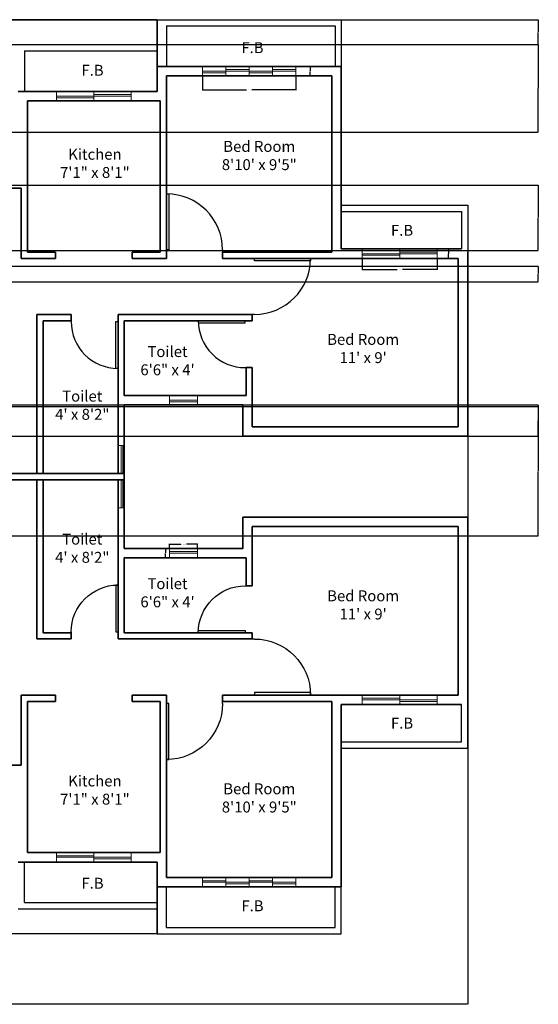
# Model space of a CAD drawing. Units: feet. Extents: x 105 to 1094, y -88 to 588.
# Tile 59 of 59: x 762 to 1094, y -88 to 543. Entities that reach past the tile are written whole.
import ezdxf

# ---------------------------------------------------------------- set-up
doc = ezdxf.new("R2010")
doc.units = ezdxf.units.FT
doc.header["$MEASUREMENT"] = 0
for name, color, linetype, lineweight in [('A-ANNO-DIMS', 2, 'Continuous', 18), ('A-ANNO-TEXT', 7, 'Continuous', 18), ('A-AREA-IDEN', 7, 'Continuous', 18), ('A-DOOR', 3, 'Continuous', 25), ('A-FLOR-PROJ', 8, 'Continuous', 25), ('A-GLAZ', 4, 'Continuous', 18), ('A-WALL', 7, 'Continuous', 35)]:
    doc.layers.add(name, color=color, linetype=linetype, lineweight=lineweight)
doc.styles.get("Standard").update_dxf_attribs({"font": 'arial.ttf'})
doc.dimstyles.get("Standard").update_dxf_attribs({"dimtxt": 0.18, "dimasz": 0.18, "dimexe": 0.18, "dimexo": 0.0625, "dimgap": 0.09, "dimtad": 0, "dimtih": 1, "dimtoh": 1, "dimdec": 4, "dimzin": 0, "dimdsep": 46, "dimtxsty": 'Standard', "dimcen": 0.09, "dimadec": 0, "dimazin": 0, "dimtfac": 1, "dimtdec": 4, "dimtofl": 0, "dimtmove": 0, "dimatfit": 3, "dimfxl": 1, "dimtolj": 1, "dimtzin": 0, "dimarcsym": 0})

# ---------------------------------------------------------------- blocks, each defined once
blk = doc.blocks.new('*U2')
for p, q in [((0, 0), (0, -6)), ((40, 0), (40, -6))]:
    blk.add_line(p, q)
blk.add_lwpolyline([(0, 0), (0, 40), (1.75, 40), (1.75, 0)], close=True)
blk.add_arc((0, 0), 40, 0, 90)
blk = doc.blocks.new('*U4')
for p, q in [((0, 0), (0, -6)), ((-40, 0), (-40, -6))]:
    blk.add_line(p, q)
blk.add_lwpolyline([(0, 0), (0, 40), (-1.75, 40), (-1.75, 0)], close=True)
blk.add_arc((0, 0), 40, 90, 180)
blk = doc.blocks.new('WIN-TWO-LIGHT')
for p, q in [((0, 0), (0, 6)), ((0, 3), (48, 3)), ((0, 2), (24, 2)), ((24, 0), (24, 6)), ((24, 4), (48, 4)), ((48, 0), (48, 6))]:
    blk.add_line(p, q)
blk = doc.blocks.new('WIN-FOUR-LIGHT')
for p, q in [((0, 0), (0, 6)), ((0, 3), (60, 3)), ((0, 2), (15, 2)), ((15, 0), (15, 6)), ((15, 4), (30, 4)), ((30, 0), (30, 6)), ((30, 2), (45, 2)), ((45, 0), (45, 6)), ((45, 4), (60, 4)), ((60, 0), (60, 6))]:
    blk.add_line(p, q)
blk = doc.blocks.new('VENT-TRANSVERSE')
for p, q in [((0, 0), (0, 6)), ((0, 3), (18, 3)), ((0, 2), (18, 2)), ((18, 0), (18, 6))]:
    blk.add_line(p, q)
blk = doc.blocks.new('VENT-LONGITUDINAL')
for p, q in [((0, 18), (4, 18)), ((2.04, 0), (2, 18)), ((3.04, 0), (3, 18))]:
    blk.add_line(p, q)
blk = doc.blocks.new('*D10')
at = {"layer": 'A-ANNO-DIMS', "color": 0, "lineweight": -2, "transparency": 16777216}
for p, q in [((981.19, 390.02), (981.19, 382.7)), ((1029.19, 390.02), (1029.19, 382.7)), ((981.37, 382.88), (1003.56, 382.88)), ((1029.01, 382.88), (1006.82, 382.88))]:
    blk.add_line(p, q, dxfattribs=at)
at = {"layer": 'A-ANNO-DIMS', "color": 0, "transparency": 16777216}
for points in [[(981.37, 382.91), (981.37, 382.85), (981.19, 382.88)], [(1029.01, 382.91), (1029.01, 382.85), (1029.19, 382.88)]]:
    blk.add_solid(points, dxfattribs=at)
at = {"layer": 'Defpoints', "color": 0, "transparency": 16777216}
for p in [(981.19, 390.08), (1029.19, 390.08), (981.19, 382.88)]:
    blk.add_point(p, dxfattribs=at)
at = {"layer": 'A-ANNO-DIMS', "color": 0, "transparency": 16777216, "insert": (1005.19, 382.88), "char_height": 0.18, "attachment_point": 5}
blk.add_mtext('\\A1;2-LIGHT WINDOW 48 TYP.', dxfattribs=at)
blk = doc.blocks.new('*D11')
at = {"layer": 'A-ANNO-DIMS', "color": 0, "lineweight": -2, "transparency": 16777216}
for p, q in [((1029.25, 396.08), (1036.57, 396.08)), ((1036.39, 395.9), (1036.39, 393.26)), ((1036.39, 390.26), (1036.39, 392.9)), ((1029.25, 390.08), (1036.57, 390.08))]:
    blk.add_line(p, q, dxfattribs=at)
at = {"layer": 'A-ANNO-DIMS', "color": 0, "transparency": 16777216}
for points in [[(1036.36, 395.9), (1036.42, 395.9), (1036.39, 396.08)], [(1036.36, 390.26), (1036.42, 390.26), (1036.39, 390.08)]]:
    blk.add_solid(points, dxfattribs=at)
at = {"layer": 'Defpoints', "color": 0, "transparency": 16777216}
for p in [(1029.19, 396.08), (1029.19, 390.08), (1036.39, 390.08)]:
    blk.add_point(p, dxfattribs=at)
at = {"layer": 'A-ANNO-DIMS', "color": 0, "transparency": 16777216, "insert": (1036.39, 393.08), "char_height": 0.18, "attachment_point": 5}
blk.add_mtext('\\A1;6 TYP.', dxfattribs=at)
blk = doc.blocks.new('*D14')
at = {"layer": 'A-ANNO-DIMS', "color": 0, "lineweight": -2, "transparency": 16777216}
for p, q in [((878.69, 507.02), (878.69, 497.9)), ((938.69, 507.02), (938.69, 497.9)), ((878.87, 498.08), (907.05, 498.08)), ((938.51, 498.08), (910.32, 498.08))]:
    blk.add_line(p, q, dxfattribs=at)
at = {"layer": 'A-ANNO-DIMS', "color": 0, "transparency": 16777216}
for points in [[(878.87, 498.11), (878.87, 498.05), (878.69, 498.08)], [(938.51, 498.11), (938.51, 498.05), (938.69, 498.08)]]:
    blk.add_solid(points, dxfattribs=at)
at = {"layer": 'Defpoints', "color": 0, "transparency": 16777216}
for p in [(878.69, 507.08), (938.69, 507.08), (938.69, 498.08)]:
    blk.add_point(p, dxfattribs=at)
at = {"layer": 'A-ANNO-DIMS', "color": 0, "transparency": 16777216, "insert": (908.69, 498.08), "char_height": 0.18, "attachment_point": 5}
blk.add_mtext('\\A1;4-LIGHT WINDOW 60 TYP.', dxfattribs=at)
blk = doc.blocks.new('*D15')
at = {"layer": 'A-ANNO-DIMS', "color": 0, "lineweight": -2, "transparency": 16777216}
for p, q in [((938.75, 513.08), (947.87, 513.08)), ((947.69, 512.9), (947.69, 510.26)), ((938.75, 507.08), (947.87, 507.08)), ((947.69, 507.26), (947.69, 509.9))]:
    blk.add_line(p, q, dxfattribs=at)
at = {"layer": 'A-ANNO-DIMS', "color": 0, "transparency": 16777216}
for points in [[(947.66, 512.9), (947.72, 512.9), (947.69, 513.08)], [(947.66, 507.26), (947.72, 507.26), (947.69, 507.08)]]:
    blk.add_solid(points, dxfattribs=at)
at = {"layer": 'Defpoints', "color": 0, "transparency": 16777216}
for p in [(938.69, 513.08), (947.69, 513.08), (938.69, 507.08)]:
    blk.add_point(p, dxfattribs=at)
at = {"layer": 'A-ANNO-DIMS', "color": 0, "transparency": 16777216, "insert": (947.69, 510.08), "char_height": 0.18, "attachment_point": 5}
blk.add_mtext('\\A1;6 TYP.', dxfattribs=at)
blk = doc.blocks.new('*D16')
at = {"layer": 'A-ANNO-DIMS', "color": 0, "lineweight": -2, "transparency": 16777216}
for p, q in [((857.69, 204.14), (857.69, 206.96)), ((857.87, 206.78), (864.9, 206.78)), ((875.51, 206.78), (868.48, 206.78)), ((875.69, 204.14), (875.69, 206.96))]:
    blk.add_line(p, q, dxfattribs=at)
at = {"layer": 'A-ANNO-DIMS', "color": 0, "transparency": 16777216}
for points in [[(857.87, 206.81), (857.87, 206.75), (857.69, 206.78)], [(875.51, 206.81), (875.51, 206.75), (875.69, 206.78)]]:
    blk.add_solid(points, dxfattribs=at)
at = {"layer": 'Defpoints', "color": 0, "transparency": 16777216}
for p in [(857.69, 206.78), (857.69, 204.08), (875.69, 204.08)]:
    blk.add_point(p, dxfattribs=at)
at = {"layer": 'A-ANNO-DIMS', "color": 0, "transparency": 16777216, "insert": (866.69, 206.78), "char_height": 0.18, "attachment_point": 5}
blk.add_mtext('\\A1;TRANSVERSE VENT 18 TYP.', dxfattribs=at)
blk = doc.blocks.new('*D17')
at = {"layer": 'A-ANNO-DIMS', "color": 0, "lineweight": -2, "transparency": 16777216}
for p, q in [((857.63, 204.08), (854.81, 204.08)), ((854.99, 203.9), (854.99, 201.26)), ((857.63, 198.08), (854.81, 198.08)), ((854.99, 198.26), (854.99, 200.9))]:
    blk.add_line(p, q, dxfattribs=at)
at = {"layer": 'A-ANNO-DIMS', "color": 0, "transparency": 16777216}
for points in [[(854.96, 203.9), (855.02, 203.9), (854.99, 204.08)], [(854.96, 198.26), (855.02, 198.26), (854.99, 198.08)]]:
    blk.add_solid(points, dxfattribs=at)
at = {"layer": 'Defpoints', "color": 0, "transparency": 16777216}
for p in [(857.69, 204.08), (854.99, 198.08), (857.69, 198.08)]:
    blk.add_point(p, dxfattribs=at)
at = {"layer": 'A-ANNO-DIMS', "color": 0, "transparency": 16777216, "insert": (854.99, 201.08), "char_height": 0.18, "attachment_point": 5}
blk.add_mtext('\\A1;6 TYP.', dxfattribs=at)
blk = doc.blocks.new('*D20')
at = {"layer": 'A-ANNO-DIMS', "color": 0, "lineweight": -2, "transparency": 16777216}
for p, q in [((150.69, 276.02), (150.69, -88.15)), ((1048.69, 276.02), (1048.69, -88.15)), ((150.87, -87.97), (599.4, -87.97)), ((1048.51, -87.97), (599.98, -87.97))]:
    blk.add_line(p, q, dxfattribs=at)
at = {"layer": 'A-ANNO-DIMS', "color": 0, "transparency": 16777216}
for points in [[(150.87, -87.94), (150.87, -88), (150.69, -87.97)], [(1048.51, -87.94), (1048.51, -88), (1048.69, -87.97)]]:
    blk.add_solid(points, dxfattribs=at)
at = {"layer": 'Defpoints', "color": 0, "transparency": 16777216}
for p in [(150.69, 276.08), (1048.69, 276.08), (1048.69, -87.97)]:
    blk.add_point(p, dxfattribs=at)
at = {"layer": 'A-ANNO-DIMS', "color": 0, "transparency": 16777216, "insert": (599.69, -87.97), "char_height": 0.18, "attachment_point": 5}
blk.add_mtext('\\A1;898', dxfattribs=at)
blk = doc.blocks.new('*D21')
at = {"layer": 'A-ANNO-DIMS', "color": 0, "lineweight": -2, "transparency": 16777216}
for p, q in [((849.63, 543.08), (105.46, 543.08)), ((105.64, 542.9), (105.64, 250.26)), ((105.64, -42.74), (105.64, 249.9)), ((849.63, -42.92), (105.46, -42.92))]:
    blk.add_line(p, q, dxfattribs=at)
at = {"layer": 'A-ANNO-DIMS', "color": 0, "transparency": 16777216}
for points in [[(105.61, 542.9), (105.67, 542.9), (105.64, 543.08)], [(105.61, -42.74), (105.67, -42.74), (105.64, -42.92)]]:
    blk.add_solid(points, dxfattribs=at)
at = {"layer": 'Defpoints', "color": 0, "transparency": 16777216}
for p in [(105.64, 543.08), (849.69, 543.08), (849.69, -42.92)]:
    blk.add_point(p, dxfattribs=at)
at = {"layer": 'A-ANNO-DIMS', "color": 0, "transparency": 16777216, "insert": (105.64, 250.08), "char_height": 0.18, "attachment_point": 5}
blk.add_mtext('\\A1;586', dxfattribs=at)
blk = doc.blocks.new('*D30')
at = {"layer": 'A-ANNO-DIMS', "color": 0, "lineweight": -2, "transparency": 16777216}
for p, q in [((349.75, 543.08), (1093.92, 543.08)), ((1093.74, 542.9), (1093.74, 535.26)), ((1093.74, 527.26), (1093.74, 534.9)), ((349.75, 527.08), (1093.92, 527.08))]:
    blk.add_line(p, q, dxfattribs=at)
at = {"layer": 'A-ANNO-DIMS', "color": 0, "transparency": 16777216}
for points in [[(1093.71, 542.9), (1093.77, 542.9), (1093.74, 543.08)], [(1093.71, 527.26), (1093.77, 527.26), (1093.74, 527.08)]]:
    blk.add_solid(points, dxfattribs=at)
at = {"layer": 'Defpoints', "color": 0, "transparency": 16777216}
for p in [(349.69, 543.08), (349.69, 527.08), (1093.74, 527.08)]:
    blk.add_point(p, dxfattribs=at)
at = {"layer": 'A-ANNO-DIMS', "color": 0, "transparency": 16777216, "insert": (1093.74, 535.08), "char_height": 0.18, "attachment_point": 5}
blk.add_mtext('\\A1;16', dxfattribs=at)
blk = doc.blocks.new('*D31')
at = {"layer": 'A-ANNO-DIMS', "color": 0, "lineweight": -2, "transparency": 16777216}
for p, q in [((438.75, 527.08), (1093.92, 527.08)), ((1093.74, 526.9), (1093.74, 499.26)), ((1093.74, 471.26), (1093.74, 498.9)), ((438.75, 471.08), (1093.92, 471.08))]:
    blk.add_line(p, q, dxfattribs=at)
at = {"layer": 'A-ANNO-DIMS', "color": 0, "transparency": 16777216}
for points in [[(1093.71, 526.9), (1093.77, 526.9), (1093.74, 527.08)], [(1093.71, 471.26), (1093.77, 471.26), (1093.74, 471.08)]]:
    blk.add_solid(points, dxfattribs=at)
at = {"layer": 'Defpoints', "color": 0, "transparency": 16777216}
for p in [(438.69, 527.08), (1093.74, 527.08), (438.69, 471.08)]:
    blk.add_point(p, dxfattribs=at)
at = {"layer": 'A-ANNO-DIMS', "color": 0, "transparency": 16777216, "insert": (1093.74, 499.08), "char_height": 0.18, "attachment_point": 5}
blk.add_mtext('\\A1;56', dxfattribs=at)
blk = doc.blocks.new('*D34')
at = {"layer": 'A-ANNO-DIMS', "color": 0, "lineweight": -2, "transparency": 16777216}
for p, q in [((552.75, 295.08), (1093.92, 295.08)), ((1093.74, 294.9), (1093.74, 253.76)), ((1093.74, 212.26), (1093.74, 253.4)), ((552.75, 212.08), (1093.92, 212.08))]:
    blk.add_line(p, q, dxfattribs=at)
at = {"layer": 'A-ANNO-DIMS', "color": 0, "transparency": 16777216}
for points in [[(1093.71, 294.9), (1093.77, 294.9), (1093.74, 295.08)], [(1093.71, 212.26), (1093.77, 212.26), (1093.74, 212.08)]]:
    blk.add_solid(points, dxfattribs=at)
at = {"layer": 'Defpoints', "color": 0, "transparency": 16777216}
for p in [(552.69, 295.08), (552.69, 212.08), (1093.74, 212.08)]:
    blk.add_point(p, dxfattribs=at)
at = {"layer": 'A-ANNO-DIMS', "color": 0, "transparency": 16777216, "insert": (1093.74, 253.58), "char_height": 0.18, "attachment_point": 5}
blk.add_mtext('\\A1;83', dxfattribs=at)
blk = doc.blocks.new('*D45')
at = {"layer": 'A-ANNO-DIMS', "color": 0, "lineweight": -2, "transparency": 16777216}
for p, q in [((552.75, 437.08), (1093.92, 437.08)), ((1093.74, 436.9), (1093.74, 416.26)), ((1093.74, 395.26), (1093.74, 415.9)), ((552.75, 395.08), (1093.92, 395.08))]:
    blk.add_line(p, q, dxfattribs=at)
at = {"layer": 'A-ANNO-DIMS', "color": 0, "transparency": 16777216}
for points in [[(1093.71, 436.9), (1093.77, 436.9), (1093.74, 437.08)], [(1093.71, 395.26), (1093.77, 395.26), (1093.74, 395.08)]]:
    blk.add_solid(points, dxfattribs=at)
at = {"layer": 'Defpoints', "color": 0, "transparency": 16777216}
for p in [(552.69, 437.08), (552.69, 395.08), (1093.74, 395.08)]:
    blk.add_point(p, dxfattribs=at)
at = {"layer": 'A-ANNO-DIMS', "color": 0, "transparency": 16777216, "insert": (1093.74, 416.08), "char_height": 0.18, "attachment_point": 5}
blk.add_mtext('\\A1;42', dxfattribs=at)
blk = doc.blocks.new('*D50')
at = {"layer": 'A-ANNO-DIMS', "color": 0, "lineweight": -2, "transparency": 16777216}
for p, q in [((552.75, 385.08), (1093.92, 385.08)), ((1093.74, 384.9), (1093.74, 380.26)), ((1093.74, 375.26), (1093.74, 379.9)), ((552.75, 375.08), (1093.92, 375.08))]:
    blk.add_line(p, q, dxfattribs=at)
at = {"layer": 'A-ANNO-DIMS', "color": 0, "transparency": 16777216}
for points in [[(1093.71, 384.9), (1093.77, 384.9), (1093.74, 385.08)], [(1093.71, 375.26), (1093.77, 375.26), (1093.74, 375.08)]]:
    blk.add_solid(points, dxfattribs=at)
at = {"layer": 'Defpoints', "color": 0, "transparency": 16777216}
for p in [(552.69, 385.08), (552.69, 375.08), (1093.74, 375.08)]:
    blk.add_point(p, dxfattribs=at)
at = {"layer": 'A-ANNO-DIMS', "color": 0, "transparency": 16777216, "insert": (1093.74, 380.08), "char_height": 0.18, "attachment_point": 5}
blk.add_mtext('\\A1;10', dxfattribs=at)
blk = doc.blocks.new('*D54')
at = {"layer": 'A-ANNO-DIMS', "color": 0, "lineweight": -2, "transparency": 16777216}
for p, q in [((294.75, 296.08), (1093.92, 296.08)), ((1093.74, 295.9), (1093.74, 286.26)), ((1093.74, 276.26), (1093.74, 285.9)), ((294.75, 276.08), (1093.92, 276.08))]:
    blk.add_line(p, q, dxfattribs=at)
at = {"layer": 'A-ANNO-DIMS', "color": 0, "transparency": 16777216}
for points in [[(1093.71, 295.9), (1093.77, 295.9), (1093.74, 296.08)], [(1093.71, 276.26), (1093.77, 276.26), (1093.74, 276.08)]]:
    blk.add_solid(points, dxfattribs=at)
at = {"layer": 'Defpoints', "color": 0, "transparency": 16777216}
for p in [(294.69, 296.08), (1093.74, 296.08), (294.69, 276.08)]:
    blk.add_point(p, dxfattribs=at)
at = {"layer": 'A-ANNO-DIMS', "color": 0, "transparency": 16777216, "insert": (1093.74, 286.08), "char_height": 0.18, "attachment_point": 5}
blk.add_mtext('\\A1;20', dxfattribs=at)

msp = doc.modelspace()

# ---------------------------------------------------------------- linework, layer by layer
at = {"layer": 'A-FLOR-PROJ'}
for p, q in [((849.6883, 543.0812), (967.6883, 543.0812)), ((967.6883, 543.0812), (967.6883, 513.0812)), ((855.6883, 539.0812), (855.6883, 513.0812)), ((855.6883, 539.0812), (963.6883, 539.0812)), ((963.6883, 539.0812), (963.6883, 513.0812)), ((760.6883, 527.0812), (849.6883, 527.0812)), ((855.6883, 527.0812), (855.6883, 513.0812)), ((764.6883, 523.0812), (849.6883, 523.0812)), ((764.6883, 523.0812), (764.6883, 497.0812)), ((967.6883, 424.0812), (1048.6883, 424.0812)), ((1048.6883, 424.0812), (1048.6883, 394.0812)), ((967.6883, 420.0812), (1044.6883, 420.0812)), ((1044.6883, 420.0812), (1044.6883, 396.0812)), ((1044.6883, 80.0812), (1044.6883, 104.0812)), ((1048.6883, 76.0812), (1048.6883, 106.0812)), ((967.6883, 80.0812), (1044.6883, 80.0812)), ((967.6883, 76.0812), (1048.6883, 76.0812)), ((764.6883, -22.9188), (764.6883, 3.0812)), ((855.6883, -38.9188), (855.6883, -12.9188)), ((855.6883, -26.9188), (855.6883, -12.9188)), ((963.6883, -38.9188), (963.6883, -12.9188)), ((967.6883, -42.9188), (967.6883, -12.9188)), ((764.6883, -22.9188), (849.6883, -22.9188)), ((760.6883, -26.9188), (849.6883, -26.9188)), ((849.6883, -42.9188), (967.6883, -42.9188)), ((855.6883, -38.9188), (963.6883, -38.9188))]:
    msp.add_line(p, q, dxfattribs=at)
at = {"layer": 'A-WALL'}
for p, q in [((849.6883, 543.0812), (849.6883, 497.0812)), ((849.6883, 513.0812), (967.6883, 513.0812)), ((967.6883, 513.0812), (967.6883, 396.0812)), ((855.6883, 507.0812), (855.6883, 390.0812)), ((855.6883, 507.0812), (961.6883, 507.0812)), ((961.6883, 507.0812), (961.6883, 394.0812)), ((760.6883, 497.0812), (849.6883, 497.0812)), ((766.6883, 491.0812), (766.6883, 394.0812)), ((766.6883, 491.0812), (851.6883, 491.0812)), ((851.6883, 491.0812), (851.6883, 394.0812)), ((762.6883, 435.0812), (652.6883, 435.0812)), ((762.6883, 435.0812), (762.6883, 390.0812)), ((766.6883, 394.0812), (784.6883, 394.0812)), ((784.6883, 394.0812), (784.6883, 390.0812)), ((833.6883, 394.0812), (833.6883, 390.0812)), ((833.6883, 394.0812), (851.6883, 394.0812)), ((891.6883, 394.0812), (891.6883, 390.0812)), ((891.6883, 394.0812), (961.6883, 394.0812)), ((967.6883, 396.0812), (1044.6883, 396.0812)), ((1048.6883, 276.0812), (1048.6883, 394.0812)), ((762.6883, 390.0812), (784.6883, 390.0812)), ((833.6883, 390.0812), (855.6883, 390.0812)), ((891.6883, 390.0812), (1042.6883, 390.0812)), ((1042.6883, 282.0812), (1042.6883, 390.0812)), ((772.6883, 252.0812), (772.6883, 354.0812)), ((772.6883, 354.0812), (794.6883, 354.0812)), ((794.6883, 350.0812), (794.6883, 354.0812)), ((824.6883, 252.0812), (824.6883, 354.0812)), ((824.6883, 354.0812), (910.6883, 354.0812)), ((910.6883, 350.0812), (910.6883, 354.0812)), ((776.6883, 252.0812), (776.6883, 350.0812)), ((776.6883, 350.0812), (794.6883, 350.0812)), ((828.6883, 302.0812), (828.6883, 350.0812)), ((828.6883, 350.0812), (910.6883, 350.0812)), ((906.6883, 302.0812), (906.6883, 320.0812)), ((906.6883, 320.0812), (910.6883, 320.0812)), ((910.6883, 282.0812), (910.6883, 320.0812)), ((828.6883, 302.0812), (906.6883, 302.0812)), ((828.6883, 248.0812), (828.6883, 296.0812)), ((828.6883, 296.0812), (904.6883, 296.0812)), ((904.6883, 276.0812), (904.6883, 296.0812)), ((910.6883, 282.0812), (1042.6883, 282.0812)), ((904.6883, 276.0812), (1048.6883, 276.0812)), ((646.6883, 252.0812), (772.6883, 252.0812)), ((646.6883, 252.0812), (828.6883, 252.0812)), ((646.6883, 248.0812), (828.6883, 248.0812)), ((646.6883, 248.0812), (772.6883, 248.0812)), ((772.6883, 248.0812), (772.6883, 146.0812)), ((776.6883, 252.0812), (828.6883, 252.0812)), ((776.6883, 248.0812), (828.6883, 248.0812)), ((776.6883, 248.0812), (776.6883, 150.0812)), ((824.6883, 248.0812), (824.6883, 146.0812)), ((828.6883, 252.0812), (828.6883, 204.0812)), ((904.6883, 224.0812), (1048.6883, 224.0812)), ((904.6883, 224.0812), (904.6883, 204.0812)), ((1048.6883, 224.0812), (1048.6883, 106.0812)), ((910.6883, 218.0812), (1042.6883, 218.0812)), ((910.6883, 218.0812), (910.6883, 180.0812)), ((1042.6883, 218.0812), (1042.6883, 110.0812)), ((828.6883, 204.0812), (904.6883, 204.0812)), ((828.6883, 198.0812), (906.6883, 198.0812)), ((828.6883, 198.0812), (828.6883, 150.0812)), ((906.6883, 198.0812), (906.6883, 180.0812)), ((906.6883, 180.0812), (910.6883, 180.0812)), ((772.6883, 146.0812), (794.6883, 146.0812)), ((776.6883, 150.0812), (794.6883, 150.0812)), ((794.6883, 150.0812), (794.6883, 146.0812)), ((824.6883, 146.0812), (910.6883, 146.0812)), ((828.6883, 150.0812), (910.6883, 150.0812)), ((910.6883, 150.0812), (910.6883, 146.0812)), ((762.6883, 110.0812), (784.6883, 110.0812)), ((762.6883, 65.0812), (762.6883, 110.0812)), ((784.6883, 106.0812), (784.6883, 110.0812)), ((833.6883, 110.0812), (855.6883, 110.0812)), ((833.6883, 106.0812), (833.6883, 110.0812)), ((855.6883, -6.9188), (855.6883, 110.0812)), ((891.6883, 110.0812), (1042.6883, 110.0812)), ((891.6883, 106.0812), (891.6883, 110.0812)), ((766.6883, 106.0812), (784.6883, 106.0812)), ((766.6883, 9.0812), (766.6883, 106.0812)), ((833.6883, 106.0812), (851.6883, 106.0812)), ((851.6883, 9.0812), (851.6883, 106.0812)), ((891.6883, 106.0812), (961.6883, 106.0812)), ((961.6883, -6.9188), (961.6883, 106.0812)), ((967.6883, 104.0812), (1044.6883, 104.0812)), ((967.6883, -12.9188), (967.6883, 104.0812)), ((762.6883, 65.0812), (652.6883, 65.0812)), ((766.6883, 9.0812), (851.6883, 9.0812)), ((760.6883, 3.0812), (849.6883, 3.0812)), ((849.6883, -42.9188), (849.6883, 3.0812)), ((855.6883, -6.9188), (961.6883, -6.9188)), ((849.6883, -12.9188), (967.6883, -12.9188))]:
    msp.add_line(p, q, dxfattribs=at)

# ---------------------------------------------------------------- block references
at = {"layer": 'A-DOOR'}
for p, xscale, yscale, zscale in [((855.6883, 395.4719), 0.8984622266767051, 0.8984622266767051, 0.8984622266767051), ((824.6883, 150.5895), -0.7513941790917756, 0.7513941790917756, 0.7513941790917756)]:
    msp.add_blockref('*U2', p, dxfattribs=dict(at, xscale=xscale, yscale=yscale, zscale=zscale))
for name, p, xscale, yscale, zscale, rotation in [('*U2', (912.0791, 390.0812), 0.8984622266767051, 0.8984622266767051, 0.8984622266767051, 270), ('*U2', (824.6883, 349.5728), 0.7513941790917756, 0.7513941790917756, 0.7513941790917756, 180), ('*U4', (906.18, 350.0812), 0.7513941790917756, 0.7513941790917756, 0.7513941790917756, 89.99999999999999), ('*U4', (906.18, 150.0812), -0.7513941790917756, 0.7513941790917756, 0.7513941790917756, 90), ('*U2', (912.0791, 110.0812), -0.8984622266767051, 0.8984622266767051, 0.8984622266767051, 270), ('*U2', (855.6883, 104.6904), -0.8984622266767051, 0.8984622266767051, 0.8984622266767051, 180)]:
    msp.add_blockref(name, p, dxfattribs=dict(at, xscale=xscale, yscale=yscale, zscale=zscale, rotation=rotation))
at = {"layer": 'A-GLAZ'}
for name, p in [('WIN-FOUR-LIGHT', (878.688, 507.081)), ('WIN-TWO-LIGHT', (785.188, 491.081)), ('VENT-TRANSVERSE', (857.688, 296.081)), ('VENT-LONGITUDINAL', (824.688, 252.081))]:
    msp.add_blockref(name, p, dxfattribs=at)
at = {"layer": 'A-GLAZ', "rotation": 180}
for name, p in [('WIN-TWO-LIGHT', (1029.1886, 396.0813)), ('VENT-TRANSVERSE', (875.6886, 204.0813))]:
    msp.add_blockref(name, p, dxfattribs=at)
at = {"layer": 'A-GLAZ', "extrusion": (0, 0, -1), "zscale": -1, "rotation": 180}
for name, p in [('VENT-LONGITUDINAL', (-824.688, 248.0813)), ('WIN-TWO-LIGHT', (-785.188, 9.0813)), ('WIN-FOUR-LIGHT', (-878.688, -6.9187))]:
    msp.add_blockref(name, p, dxfattribs=at)
at = {"layer": 'A-GLAZ', "extrusion": (0, 0, -1), "zscale": -1}
msp.add_blockref('WIN-TWO-LIGHT', (-1029.1886, 104.081), dxfattribs=at)

# ---------------------------------------------------------------- texts
at = {"layer": 'A-ANNO-TEXT', "char_height": 7}
for insert, attachment_point in [((861.6308, 528.6595), 1), ((759.1716, 514.1723), 1), ((957.4727, 411.5608), 1), ((957.4727, 88.6015), 7), ((759.1716, -14.01), 7), ((861.6308, -28.4972), 7)]:
    msp.add_mtext_dynamic_manual_height_columns('\\pxqc;F.B ', width=98.34246, gutter_width=1, heights=[0], dxfattribs=dict(at, insert=insert, attachment_point=attachment_point))
at = {"layer": 'A-AREA-IDEN', "char_height": 7}
for s, insert, attachment_point in [('\\pxqc;Kitchen  \\P7\'1" x 8\'1"', (760.6883, 460.3027), 1), ('\\pxqc;Bed Room \\P8\'10\' x 9\'5"', (865.9929, 465.329), 1), ("\\pxqc;Bed Room \\P11' x 9'", (932.5509, 341.6038), 1), ('\\pxqc;Toilet \\P6\'6" x 4\'', (807.2162, 333.8075), 1), ('\\pxqc;Toilet \\P4\' x 8\'2"', (752.6121, 305.2595), 1), ('\\pxqc;Toilet \\P4\' x 8\'2"', (752.6121, 194.9029), 7), ('\\pxqc;Toilet \\P6\'6" x 4\'', (807.2162, 166.3548), 7), ("\\pxqc;Bed Room \\P11' x 9'", (932.5509, 158.5586), 7), ('\\pxqc;Kitchen  \\P7\'1" x 8\'1"', (760.6883, 39.8597), 7), ('\\pxqc;Bed Room \\P8\'10\' x 9\'5"', (865.9929, 34.8333), 7)]:
    msp.add_mtext_dynamic_manual_height_columns(s, width=98.34246, gutter_width=1, heights=[0], dxfattribs=dict(at, insert=insert, attachment_point=attachment_point))

# ---------------------------------------------------------------- dimensions: what is measured, and where the dimension line sits
at = {"layer": 'A-ANNO-DIMS'}
for base, p1, p2, picture, middle in [((105.6383, 543.0812), (849.6883, -42.9188), (849.6883, 543.0812), '*D21', (105.6383, 250.0812)), ((1093.7383, 527.0812), (349.6883, 543.0812), (349.6883, 527.0812), '*D30', (1093.7383, 535.0812)), ((1093.7383, 527.0812), (438.6883, 471.0812), (438.6883, 527.0812), '*D31', (1093.7383, 499.0812)), ((1093.7383, 395.0812), (552.6883, 437.0812), (552.6883, 395.0812), '*D45', (1093.7383, 416.0812)), ((1093.7383, 375.0812), (552.6883, 385.0812), (552.6883, 375.0812), '*D50', (1093.7383, 380.0812)), ((1093.7383, 296.0812), (294.6883, 276.0812), (294.6883, 296.0812), '*D54', (1093.7383, 286.0812)), ((1093.7383, 212.0812), (552.6883, 295.0812), (552.6883, 212.0812), '*D34', (1093.7383, 253.5812))]:
    dim = msp.add_linear_dim(base=base, p1=p1, p2=p2, angle=90, dimstyle='Standard', override={"dimdec": 0, "dimlfac": 1, "dimrnd": 0, "dimzin": 0, "dimdsep": 46, "dimlunit": 2}, dxfattribs=at)
    dim.commit()
    dim.dimension.update_dxf_attribs({"geometry": picture, "text_midpoint": middle})
for base, p1, p2, angle, text, picture, middle in [((947.6883, 513.0812), (938.6883, 507.0812), (938.6883, 513.0812), 90, '<> TYP.', '*D15', (947.6883, 510.0812)), ((1036.3883, 390.0812), (1029.1883, 396.0812), (1029.1883, 390.0812), 270, '<> TYP.', '*D11', (1036.3883, 393.0812)), ((981.1883, 382.8812), (1029.1883, 390.0812), (981.1883, 390.0812), 180, '2-LIGHT WINDOW <> TYP.', '*D10', (1005.1883, 382.8812)), ((854.9883, 198.0812), (857.6883, 204.0812), (857.6883, 198.0812), 270, '<> TYP.', '*D17', (854.9883, 201.0812)), ((857.6883, 206.7812), (875.6883, 204.0812), (857.6883, 204.0812), 180, 'TRANSVERSE VENT <> TYP.', '*D16', (866.6883, 206.7812))]:
    dim = msp.add_linear_dim(base=base, p1=p1, p2=p2, angle=angle, text=text, dimstyle='Standard', override={"dimdec": 0, "dimlfac": 1, "dimrnd": 0, "dimzin": 0, "dimdsep": 46, "dimlunit": 2}, dxfattribs=at)
    dim.commit()
    dim.dimension.update_dxf_attribs({"geometry": picture, "text_midpoint": middle})
dim = msp.add_linear_dim(base=(938.6883, 498.0812), p1=(878.6883, 507.0812), p2=(938.6883, 507.0812), text='4-LIGHT WINDOW <> TYP.', dimstyle='Standard', override={"dimdec": 0, "dimlfac": 1, "dimrnd": 0, "dimzin": 0, "dimdsep": 46, "dimlunit": 2}, dxfattribs=at)
dim.commit()
dim.dimension.update_dxf_attribs({"geometry": '*D14', "text_midpoint": (908.6883, 498.0812)})
dim = msp.add_linear_dim(base=(1048.6883, -87.9688), p1=(150.6883, 276.0812), p2=(1048.6883, 276.0812), dimstyle='Standard', override={"dimdec": 0, "dimlfac": 1, "dimrnd": 0, "dimzin": 0, "dimdsep": 46, "dimlunit": 2}, dxfattribs=at)
dim.commit()
dim.dimension.update_dxf_attribs({"geometry": '*D20', "text_midpoint": (599.6883, -87.9688)})

doc.saveas('drawing.dxf')
